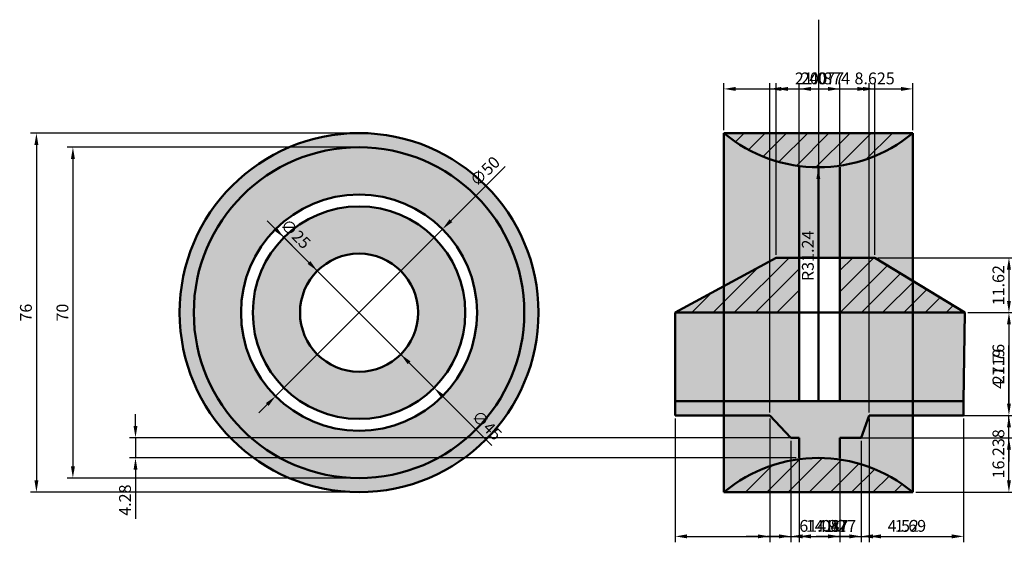
# Model space of a CAD drawing. Units: millimetres. Extents: x 1248 to 2192, y 1962 to 2325.
# Tile 1 of 4: x 1249 to 1457, y 1962 to 2073. Entities that reach past the tile are written whole.
import ezdxf

# ---------------------------------------------------------------- set-up
doc = ezdxf.new("R2010")
doc.units = ezdxf.units.MM
for name, color, linetype, lineweight in [('M-DIMS', 2, 'Continuous', 25), ('M-HATC', 8, 'Continuous', 18), ('M-OUTL', 7, 'Continuous', 50)]:
    doc.layers.add(name, color=color, linetype=linetype, lineweight=lineweight)
doc.styles.get("Standard").update_dxf_attribs({"font": 'arial.ttf'})
doc.dimstyles.new('ISO-25', dxfattribs={"dimtxt": 2.5, "dimasz": 2.5, "dimexe": 1.25, "dimexo": 0.625, "dimtad": 1, "dimtxsty": 'Standard', "dimcen": 2.5, "dimadec": 0, "dimazin": 0, "dimtfac": 1, "dimtmove": 0, "dimatfit": 3, "dimfxl": 1, "dimarcsym": 0})

# ---------------------------------------------------------------- blocks, each defined once
blk = doc.blocks.new('*D10')
at = {"layer": 'Defpoints', "color": 0, "transparency": 16777216}
for p in [(1320.58, 2048.72), (1252.24, 1972.72), (1320.58, 1972.72)]:
    blk.add_point(p, dxfattribs=at)
at = {"layer": 'M-DIMS', "color": 0, "lineweight": -2, "transparency": 16777216}
for p, q in [((1319.95, 2048.72), (1250.99, 2048.72)), ((1252.24, 2046.22), (1252.24, 1975.22)), ((1319.95, 1972.72), (1250.99, 1972.72))]:
    blk.add_line(p, q, dxfattribs=at)
at = {"layer": 'M-DIMS', "color": 0, "transparency": 16777216}
for points in [[(1251.82, 2046.22), (1252.66, 2046.22), (1252.24, 2048.72)], [(1251.82, 1975.22), (1252.66, 1975.22), (1252.24, 1972.72)]]:
    blk.add_solid(points, dxfattribs=at)
at = {"layer": 'M-DIMS', "color": 0, "transparency": 16777216, "insert": (1250.34, 2010.72), "char_height": 2.5, "attachment_point": 5, "rotation": 90}
blk.add_mtext('76', dxfattribs=at)
blk = doc.blocks.new('*D11')
at = {"layer": 'Defpoints', "color": 0, "transparency": 16777216}
for p in [(1320.58, 2045.72), (1259.97, 1975.72), (1320.58, 1975.72)]:
    blk.add_point(p, dxfattribs=at)
at = {"layer": 'M-DIMS', "color": 0, "lineweight": -2, "transparency": 16777216}
for p, q in [((1319.95, 2045.72), (1258.72, 2045.72)), ((1259.97, 2043.22), (1259.97, 1978.22)), ((1319.95, 1975.72), (1258.72, 1975.72))]:
    blk.add_line(p, q, dxfattribs=at)
at = {"layer": 'M-DIMS', "color": 0, "transparency": 16777216}
for points in [[(1259.55, 2043.22), (1260.39, 2043.22), (1259.97, 2045.72)], [(1259.55, 1978.22), (1260.39, 1978.22), (1259.97, 1975.72)]]:
    blk.add_solid(points, dxfattribs=at)
at = {"layer": 'M-DIMS', "color": 0, "transparency": 16777216, "insert": (1258.07, 2010.72), "char_height": 2.5, "attachment_point": 5, "rotation": 90}
blk.add_mtext('70', dxfattribs=at)
blk = doc.blocks.new('*D41')
at = {"layer": 'Defpoints', "color": 0, "transparency": 16777216}
for p in [(1437.87, 2058.07), (1397.87, 2048.72), (1437.87, 2048.72)]:
    blk.add_point(p, dxfattribs=at)
at = {"layer": 'M-DIMS', "color": 0, "lineweight": -2, "transparency": 16777216}
for p, q in [((1397.87, 2049.34), (1397.87, 2059.32)), ((1437.87, 2049.34), (1437.87, 2059.32)), ((1400.37, 2058.07), (1435.37, 2058.07))]:
    blk.add_line(p, q, dxfattribs=at)
at = {"layer": 'M-DIMS', "color": 0, "transparency": 16777216}
for points in [[(1400.37, 2058.49), (1400.37, 2057.65), (1397.87, 2058.07)], [(1435.37, 2058.49), (1435.37, 2057.65), (1437.87, 2058.07)]]:
    blk.add_solid(points, dxfattribs=at)
at = {"layer": 'M-DIMS', "color": 0, "transparency": 16777216, "insert": (1417.87, 2059.97), "char_height": 2.5, "attachment_point": 5}
blk.add_mtext('40', dxfattribs=at)
blk = doc.blocks.new('*D42')
at = {"layer": 'Defpoints', "color": 0, "transparency": 16777216}
for p in [(1387.56, 1988.96), (1448.64, 1988.96), (1448.64, 1963.37)]:
    blk.add_point(p, dxfattribs=at)
at = {"layer": 'M-DIMS', "color": 0, "lineweight": -2, "transparency": 16777216}
for p, q in [((1387.56, 1988.33), (1387.56, 1962.12)), ((1448.64, 1988.33), (1448.64, 1962.12)), ((1390.06, 1963.37), (1446.14, 1963.37))]:
    blk.add_line(p, q, dxfattribs=at)
at = {"layer": 'M-DIMS', "color": 0, "transparency": 16777216}
for points in [[(1390.06, 1963.79), (1390.06, 1962.95), (1387.56, 1963.37)], [(1446.14, 1963.79), (1446.14, 1962.95), (1448.64, 1963.37)]]:
    blk.add_solid(points, dxfattribs=at)
at = {"layer": 'M-DIMS', "color": 0, "transparency": 16777216, "insert": (1418.1, 1965.27), "char_height": 2.5, "attachment_point": 5}
blk.add_mtext('61.08', dxfattribs=at)
blk = doc.blocks.new('*D43')
at = {"layer": 'Defpoints', "color": 0, "transparency": 16777216}
for p in [(1448.89, 2010.72), (1448.64, 1988.96), (1458.24, 1988.96)]:
    blk.add_point(p, dxfattribs=at)
at = {"layer": 'M-DIMS', "color": 0, "lineweight": -2, "transparency": 16777216}
for p, q in [((1449.52, 2010.72), (1459.49, 2010.72)), ((1458.24, 2008.22), (1458.24, 1991.46)), ((1449.26, 1988.96), (1459.49, 1988.96))]:
    blk.add_line(p, q, dxfattribs=at)
at = {"layer": 'M-DIMS', "color": 0, "transparency": 16777216}
for points in [[(1457.83, 2008.22), (1458.66, 2008.22), (1458.24, 2010.72)], [(1457.83, 1991.46), (1458.66, 1991.46), (1458.24, 1988.96)]]:
    blk.add_solid(points, dxfattribs=at)
at = {"layer": 'M-DIMS', "color": 0, "transparency": 16777216, "insert": (1456.34, 1999.84), "char_height": 2.5, "attachment_point": 5, "rotation": 90}
blk.add_mtext('21.76', dxfattribs=at)
blk = doc.blocks.new('*D44')
at = {"layer": 'Defpoints', "color": 0, "transparency": 16777216}
for p in [(1429.82, 2022.34), (1448.89, 2010.72), (1458.24, 2010.72)]:
    blk.add_point(p, dxfattribs=at)
at = {"layer": 'M-DIMS', "color": 0, "lineweight": -2, "transparency": 16777216}
for p, q in [((1430.45, 2022.34), (1459.49, 2022.34)), ((1458.24, 2019.84), (1458.24, 2013.22)), ((1449.52, 2010.72), (1459.49, 2010.72))]:
    blk.add_line(p, q, dxfattribs=at)
at = {"layer": 'M-DIMS', "color": 0, "transparency": 16777216}
for points in [[(1457.83, 2019.84), (1458.66, 2019.84), (1458.24, 2022.34)], [(1457.83, 2013.22), (1458.66, 2013.22), (1458.24, 2010.72)]]:
    blk.add_solid(points, dxfattribs=at)
at = {"layer": 'M-DIMS', "color": 0, "transparency": 16777216, "insert": (1456.34, 2016.53), "char_height": 2.5, "attachment_point": 5, "rotation": 90}
blk.add_mtext('11.62', dxfattribs=at)
blk = doc.blocks.new('*D45')
at = {"layer": 'Defpoints', "color": 0, "transparency": 16777216}
for p in [(1448.64, 1988.96), (1458.24, 1988.96), (1437.87, 1972.72)]:
    blk.add_point(p, dxfattribs=at)
at = {"layer": 'M-DIMS', "color": 0, "lineweight": -2, "transparency": 16777216}
for p, q in [((1449.26, 1988.96), (1459.49, 1988.96)), ((1458.24, 1975.22), (1458.24, 1986.46)), ((1438.49, 1972.72), (1459.49, 1972.72))]:
    blk.add_line(p, q, dxfattribs=at)
at = {"layer": 'M-DIMS', "color": 0, "transparency": 16777216}
for points in [[(1457.83, 1986.46), (1458.66, 1986.46), (1458.24, 1988.96)], [(1457.83, 1975.22), (1458.66, 1975.22), (1458.24, 1972.72)]]:
    blk.add_solid(points, dxfattribs=at)
at = {"layer": 'M-DIMS', "color": 0, "transparency": 16777216, "insert": (1456.34, 1980.84), "char_height": 2.5, "attachment_point": 5, "rotation": 90}
blk.add_mtext('16.238', dxfattribs=at)
blk = doc.blocks.new('*D46')
at = {"layer": 'Defpoints', "color": 0, "transparency": 16777216}
for p in [(1429.82, 2058.07), (1408.95, 2022.34), (1429.82, 2022.34)]:
    blk.add_point(p, dxfattribs=at)
at = {"layer": 'M-DIMS', "color": 0, "lineweight": -2, "transparency": 16777216}
for p, q in [((1408.95, 2022.97), (1408.95, 2059.32)), ((1429.82, 2022.97), (1429.82, 2059.32)), ((1411.45, 2058.07), (1427.32, 2058.07))]:
    blk.add_line(p, q, dxfattribs=at)
at = {"layer": 'M-DIMS', "color": 0, "transparency": 16777216}
for points in [[(1411.45, 2058.49), (1411.45, 2057.65), (1408.95, 2058.07)], [(1427.32, 2058.49), (1427.32, 2057.65), (1429.82, 2058.07)]]:
    blk.add_solid(points, dxfattribs=at)
at = {"layer": 'M-DIMS', "color": 0, "transparency": 16777216, "insert": (1419.39, 2059.97), "char_height": 2.5, "attachment_point": 5}
blk.add_mtext('20.874', dxfattribs=at)
blk = doc.blocks.new('*D47')
at = {"layer": 'Defpoints', "color": 0, "transparency": 16777216}
for p in [(1422.43, 2058.07), (1413.81, 2041.48), (1422.43, 2041.48)]:
    blk.add_point(p, dxfattribs=at)
at = {"layer": 'M-DIMS', "color": 0, "lineweight": -2, "transparency": 16777216}
for p, q in [((1413.81, 2042.1), (1413.81, 2059.32)), ((1422.43, 2042.1), (1422.43, 2059.32)), ((1416.31, 2058.07), (1419.93, 2058.07)), ((1422.43, 2058.07), (1434.64, 2058.07))]:
    blk.add_line(p, q, dxfattribs=at)
at = {"layer": 'M-DIMS', "color": 0, "transparency": 16777216}
for points in [[(1416.31, 2058.49), (1416.31, 2057.65), (1413.81, 2058.07)], [(1419.93, 2058.49), (1419.93, 2057.65), (1422.43, 2058.07)]]:
    blk.add_solid(points, dxfattribs=at)
at = {"layer": 'M-DIMS', "color": 0, "transparency": 16777216, "insert": (1429.79, 2059.97), "char_height": 2.5, "attachment_point": 5}
blk.add_mtext('8.625', dxfattribs=at)
blk = doc.blocks.new('*D48')
at = {"layer": 'Defpoints', "color": 0, "transparency": 16777216}
for p in [(1412.03, 1984.24), (1426.95, 1984.24), (1426.95, 1963.37)]:
    blk.add_point(p, dxfattribs=at)
at = {"layer": 'M-DIMS', "color": 0, "lineweight": -2, "transparency": 16777216}
for p, q in [((1412.03, 1983.61), (1412.03, 1962.12)), ((1426.95, 1983.61), (1426.95, 1962.12)), ((1414.53, 1963.37), (1424.45, 1963.37))]:
    blk.add_line(p, q, dxfattribs=at)
at = {"layer": 'M-DIMS', "color": 0, "transparency": 16777216}
for points in [[(1414.53, 1963.79), (1414.53, 1962.95), (1412.03, 1963.37)], [(1424.45, 1963.79), (1424.45, 1962.95), (1426.95, 1963.37)]]:
    blk.add_solid(points, dxfattribs=at)
at = {"layer": 'M-DIMS', "color": 0, "transparency": 16777216, "insert": (1419.49, 1965.27), "char_height": 2.5, "attachment_point": 5}
blk.add_mtext('14.92', dxfattribs=at)
blk = doc.blocks.new('*D49')
at = {"layer": 'Defpoints', "color": 0, "transparency": 16777216}
for p in [(1428.64, 1988.96), (1458.24, 1988.96), (1422.43, 1984.24)]:
    blk.add_point(p, dxfattribs=at)
at = {"layer": 'M-DIMS', "color": 0, "lineweight": -2, "transparency": 16777216}
for p, q in [((1458.24, 1991.46), (1458.24, 2003.75)), ((1429.26, 1988.96), (1459.49, 1988.96)), ((1458.24, 1984.24), (1458.24, 1988.96)), ((1423.06, 1984.24), (1459.49, 1984.24)), ((1458.24, 1981.74), (1458.24, 1979.24))]:
    blk.add_line(p, q, dxfattribs=at)
at = {"layer": 'M-DIMS', "color": 0, "transparency": 16777216}
for points in [[(1457.83, 1991.46), (1458.66, 1991.46), (1458.24, 1988.96)], [(1457.83, 1981.74), (1458.66, 1981.74), (1458.24, 1984.24)]]:
    blk.add_solid(points, dxfattribs=at)
at = {"layer": 'M-DIMS', "color": 0, "transparency": 16777216, "insert": (1456.34, 1998.85), "char_height": 2.5, "attachment_point": 5, "rotation": 90}
blk.add_mtext('4.719', dxfattribs=at)
blk = doc.blocks.new('*D61')
at = {"layer": 'Defpoints', "color": 0, "transparency": 16777216}
for p in [(1338.26, 2028.4), (1302.9, 1993.04)]:
    blk.add_point(p, dxfattribs=at)
at = {"layer": 'M-DIMS', "color": 0, "lineweight": -2, "transparency": 16777216}
for p, q in [((1351.53, 2041.67), (1340.02, 2030.16)), ((1302.9, 1993.04), (1338.26, 2028.4)), ((1301.13, 1991.28), (1299.36, 1989.51))]:
    blk.add_line(p, q, dxfattribs=at)
at = {"layer": 'M-DIMS', "color": 0, "transparency": 16777216}
for points in [[(1339.73, 2030.46), (1340.32, 2029.87), (1338.26, 2028.4)], [(1300.83, 1991.57), (1301.42, 1990.98), (1302.9, 1993.04)]]:
    blk.add_solid(points, dxfattribs=at)
at = {"layer": 'M-DIMS', "color": 0, "transparency": 16777216, "insert": (1347.47, 2040.4), "char_height": 2.5, "attachment_point": 5, "rotation": 44.9946}
blk.add_mtext('∅50', dxfattribs=at)
blk = doc.blocks.new('*D62')
at = {"layer": 'Defpoints', "color": 0, "transparency": 16777216}
for p in [(1304.66, 2026.63), (1336.49, 1994.81)]:
    blk.add_point(p, dxfattribs=at)
at = {"layer": 'M-DIMS', "color": 0, "lineweight": -2, "transparency": 16777216}
for p, q in [((1302.9, 2028.4), (1301.13, 2030.16)), ((1304.66, 2026.63), (1336.49, 1994.81)), ((1348.71, 1982.59), (1338.26, 1993.04))]:
    blk.add_line(p, q, dxfattribs=at)
at = {"layer": 'M-DIMS', "color": 0, "transparency": 16777216}
for points in [[(1303.19, 2028.69), (1302.6, 2028.1), (1304.66, 2026.63)], [(1338.55, 1993.34), (1337.96, 1992.75), (1336.49, 1994.81)]]:
    blk.add_solid(points, dxfattribs=at)
at = {"layer": 'M-DIMS', "color": 0, "transparency": 16777216, "insert": (1347.43, 1986.66), "char_height": 2.5, "attachment_point": 5, "rotation": 315.0063}
blk.add_mtext('∅45', dxfattribs=at)
blk = doc.blocks.new('*D63')
at = {"layer": 'Defpoints', "color": 0, "transparency": 16777216}
for p in [(1311.74, 2019.56), (1329.41, 2001.88)]:
    blk.add_point(p, dxfattribs=at)
at = {"layer": 'M-DIMS', "color": 0, "lineweight": -2, "transparency": 16777216}
for p, q in [((1302.85, 2028.45), (1309.97, 2021.33)), ((1329.41, 2001.88), (1311.74, 2019.56)), ((1331.18, 2000.11), (1332.95, 1998.34))]:
    blk.add_line(p, q, dxfattribs=at)
at = {"layer": 'M-DIMS', "color": 0, "transparency": 16777216}
for points in [[(1310.27, 2021.62), (1309.68, 2021.03), (1311.74, 2019.56)], [(1331.48, 2000.41), (1330.89, 1999.82), (1329.41, 2001.88)]]:
    blk.add_solid(points, dxfattribs=at)
at = {"layer": 'M-DIMS', "color": 0, "transparency": 16777216, "insert": (1306.92, 2027.17), "char_height": 2.5, "attachment_point": 5, "rotation": 314.9886}
blk.add_mtext('∅25', dxfattribs=at)
blk = doc.blocks.new('*D64')
at = {"layer": 'Defpoints', "color": 0, "transparency": 16777216}
for p in [(1417.87, 2072.72), (1417.87, 2041.48)]:
    blk.add_point(p, dxfattribs=at)
at = {"layer": 'M-DIMS', "color": 0, "lineweight": -2, "transparency": 16777216}
for p, q in [((1417.87, 2072.72), (1417.87, 2041.48)), ((1417.87, 2016.7), (1417.87, 2038.98))]:
    blk.add_line(p, q, dxfattribs=at)
at = {"layer": 'M-DIMS', "color": 0, "transparency": 16777216}
blk.add_solid([(1417.45, 2038.98), (1418.28, 2038.98), (1417.87, 2041.48)], dxfattribs=at)
at = {"layer": 'M-DIMS', "color": 0, "transparency": 16777216, "insert": (1415.97, 2022.74), "char_height": 2.5, "attachment_point": 5, "rotation": 89.9997}
blk.add_mtext('R31.24', dxfattribs=at)
blk = doc.blocks.new('*D69')
at = {"layer": 'Defpoints', "color": 0, "transparency": 16777216}
for p in [(1428.64, 2058.07), (1407.56, 1988.96), (1428.64, 1988.96)]:
    blk.add_point(p, dxfattribs=at)
at = {"layer": 'M-DIMS', "color": 0, "lineweight": -2, "transparency": 16777216}
for p, q in [((1407.56, 1989.58), (1407.56, 2059.32)), ((1428.64, 1989.58), (1428.64, 2059.32)), ((1410.06, 2058.07), (1426.14, 2058.07))]:
    blk.add_line(p, q, dxfattribs=at)
at = {"layer": 'M-DIMS', "color": 0, "transparency": 16777216}
for points in [[(1410.06, 2058.49), (1410.06, 2057.65), (1407.56, 2058.07)], [(1426.14, 2058.49), (1426.14, 2057.65), (1428.64, 2058.07)]]:
    blk.add_solid(points, dxfattribs=at)
at = {"layer": 'M-DIMS', "color": 0, "transparency": 16777216, "insert": (1418.1, 2059.97), "char_height": 2.5, "attachment_point": 5}
blk.add_mtext('21.077', dxfattribs=at)
blk = doc.blocks.new('*D70')
at = {"layer": 'Defpoints', "color": 0, "transparency": 16777216}
for p in [(1407.56, 1988.96), (1412.03, 1984.24), (1412.03, 1963.37)]:
    blk.add_point(p, dxfattribs=at)
at = {"layer": 'M-DIMS', "color": 0, "lineweight": -2, "transparency": 16777216}
for p, q in [((1407.56, 1988.33), (1407.56, 1962.12)), ((1412.03, 1983.61), (1412.03, 1962.12)), ((1405.06, 1963.37), (1402.56, 1963.37)), ((1407.56, 1963.37), (1412.03, 1963.37)), ((1414.53, 1963.37), (1424.88, 1963.37))]:
    blk.add_line(p, q, dxfattribs=at)
at = {"layer": 'M-DIMS', "color": 0, "transparency": 16777216}
for points in [[(1405.06, 1963.79), (1405.06, 1962.95), (1407.56, 1963.37)], [(1414.53, 1963.79), (1414.53, 1962.95), (1412.03, 1963.37)]]:
    blk.add_solid(points, dxfattribs=at)
at = {"layer": 'M-DIMS', "color": 0, "transparency": 16777216, "insert": (1420.95, 1965.24), "char_height": 2.5, "attachment_point": 5}
blk.add_mtext('4.47', dxfattribs=at)
blk = doc.blocks.new('*D71')
at = {"layer": 'Defpoints', "color": 0, "transparency": 16777216}
for p in [(1412.03, 1984.24), (1413.81, 1984.24), (1413.81, 1963.37)]:
    blk.add_point(p, dxfattribs=at)
at = {"layer": 'M-DIMS', "color": 0, "lineweight": -2, "transparency": 16777216}
for p, q in [((1412.03, 1983.61), (1412.03, 1962.12)), ((1413.81, 1983.61), (1413.81, 1962.12)), ((1409.53, 1963.37), (1407.03, 1963.37)), ((1412.03, 1963.37), (1413.81, 1963.37)), ((1416.31, 1963.37), (1426.31, 1963.37))]:
    blk.add_line(p, q, dxfattribs=at)
at = {"layer": 'M-DIMS', "color": 0, "transparency": 16777216}
for points in [[(1409.53, 1963.79), (1409.53, 1962.95), (1412.03, 1963.37)], [(1416.31, 1963.79), (1416.31, 1962.95), (1413.81, 1963.37)]]:
    blk.add_solid(points, dxfattribs=at)
at = {"layer": 'M-DIMS', "color": 0, "transparency": 16777216, "insert": (1422.56, 1965.25), "char_height": 2.5, "attachment_point": 5}
blk.add_mtext('1.77', dxfattribs=at)
blk = doc.blocks.new('*D72')
at = {"layer": 'Defpoints', "color": 0, "transparency": 16777216}
for p in [(1422.43, 1984.24), (1426.95, 1984.24), (1426.95, 1963.37)]:
    blk.add_point(p, dxfattribs=at)
at = {"layer": 'M-DIMS', "color": 0, "lineweight": -2, "transparency": 16777216}
for p, q in [((1422.43, 1983.61), (1422.43, 1962.12)), ((1426.95, 1983.61), (1426.95, 1962.12)), ((1419.93, 1963.37), (1417.43, 1963.37)), ((1422.43, 1963.37), (1426.95, 1963.37)), ((1429.45, 1963.37), (1439.77, 1963.37))]:
    blk.add_line(p, q, dxfattribs=at)
at = {"layer": 'M-DIMS', "color": 0, "transparency": 16777216}
for points in [[(1419.93, 1963.79), (1419.93, 1962.95), (1422.43, 1963.37)], [(1429.45, 1963.79), (1429.45, 1962.95), (1426.95, 1963.37)]]:
    blk.add_solid(points, dxfattribs=at)
at = {"layer": 'M-DIMS', "color": 0, "transparency": 16777216, "insert": (1435.86, 1965.27), "char_height": 2.5, "attachment_point": 5}
blk.add_mtext('4.52', dxfattribs=at)
blk = doc.blocks.new('*D73')
at = {"layer": 'Defpoints', "color": 0, "transparency": 16777216}
for p in [(1428.64, 1988.96), (1426.95, 1984.24), (1428.64, 1963.37)]:
    blk.add_point(p, dxfattribs=at)
at = {"layer": 'M-DIMS', "color": 0, "lineweight": -2, "transparency": 16777216}
for p, q in [((1428.64, 1988.33), (1428.64, 1962.12)), ((1426.95, 1983.61), (1426.95, 1962.12)), ((1424.45, 1963.37), (1421.95, 1963.37)), ((1426.95, 1963.37), (1428.64, 1963.37)), ((1431.14, 1963.37), (1441.15, 1963.37))]:
    blk.add_line(p, q, dxfattribs=at)
at = {"layer": 'M-DIMS', "color": 0, "transparency": 16777216}
for points in [[(1424.45, 1963.79), (1424.45, 1962.95), (1426.95, 1963.37)], [(1431.14, 1963.79), (1431.14, 1962.95), (1428.64, 1963.37)]]:
    blk.add_solid(points, dxfattribs=at)
at = {"layer": 'M-DIMS', "color": 0, "transparency": 16777216, "insert": (1437.39, 1965.27), "char_height": 2.5, "attachment_point": 5}
blk.add_mtext('1.69', dxfattribs=at)
blk = doc.blocks.new('*D74')
at = {"layer": 'Defpoints', "color": 0, "transparency": 16777216}
for p in [(1413.81, 1984.24), (1273.23, 1979.96), (1413.81, 1979.96)]:
    blk.add_point(p, dxfattribs=at)
at = {"layer": 'M-DIMS', "color": 0, "lineweight": -2, "transparency": 16777216}
for p, q in [((1273.23, 1986.74), (1273.23, 1989.24)), ((1413.18, 1984.24), (1271.98, 1984.24)), ((1273.23, 1984.24), (1273.23, 1979.96)), ((1413.18, 1979.96), (1271.98, 1979.96)), ((1273.23, 1977.46), (1273.23, 1967.11))]:
    blk.add_line(p, q, dxfattribs=at)
at = {"layer": 'M-DIMS', "color": 0, "transparency": 16777216}
for points in [[(1272.81, 1986.74), (1273.64, 1986.74), (1273.23, 1984.24)], [(1272.81, 1977.46), (1273.64, 1977.46), (1273.23, 1979.96)]]:
    blk.add_solid(points, dxfattribs=at)
at = {"layer": 'M-DIMS', "color": 0, "transparency": 16777216, "insert": (1271.33, 1971.04), "char_height": 2.5, "attachment_point": 5, "rotation": 90}
blk.add_mtext('4.28', dxfattribs=at)

msp = doc.modelspace()

# ---------------------------------------------------------------- hatches: boundary and pattern name
at = {"layer": 'M-HATC'}
h = msp.add_hatch(color=256, dxfattribs=at)
h.set_gradient(color1=(255, 0, 0), color2=(255, 0, 0))
h.paths.add_polyline_path([(1285.5766, 2010.7199, 1), (1355.5766, 2010.7199, 1)], flags=0)
h.paths.add_polyline_path([(1345.5766, 2010.7199, -1), (1295.5766, 2010.7199, -1)], flags=0)
h.paths.add_polyline_path([(1343.0766, 2010.7199, -1), (1298.0766, 2010.7199, -1)], flags=0)
h.paths.add_polyline_path([(1333.0766, 2010.7199, -1), (1308.0766, 2010.7199, -1)], flags=0)
h.paths.add_polyline_path([(1282.5766, 2010.7199, 1), (1358.5766, 2010.7199, 1)])
h.paths.add_polyline_path([(1355.5766, 2010.7199, -1), (1285.5766, 2010.7199, -1)], flags=16)
h = msp.add_hatch(dxfattribs=at)
h.set_pattern_fill('ANSI31', color=256)
h.paths.add_polyline_path([(1437.8682, 2048.7199), (1397.8682, 2048.7199, 0.36209663)])
h.paths.add_polyline_path([(1397.8682, 1972.7199), (1437.8682, 1972.7199, 0.362065)])
h.paths.add_polyline_path([(1413.8061, 2022.341), (1408.9497, 2022.341), (1397.8682, 2016.3204), (1397.8682, 2010.7199), (1413.8061, 2010.7199)])
h.paths.add_polyline_path([(1437.8682, 2017.4391), (1429.824, 2022.341), (1422.4308, 2022.341), (1422.4308, 2010.7199), (1437.8682, 2010.7199)])
h.paths.add_polyline_path([(1437.8682, 2017.4391), (1437.8682, 2010.7199), (1448.8945, 2010.7199)])
h.paths.add_polyline_path([(1397.8682, 2016.3204), (1387.5598, 2010.7199), (1397.8682, 2010.7199)])
h = msp.add_hatch(color=256, dxfattribs=at)
h.set_gradient(color1=(255, 0, 0), color2=(255, 0, 0))
h.paths.add_polyline_path([(1437.8682, 2048.7199), (1397.8682, 2048.7199, 0.36209663)])
h.paths.add_polyline_path([(1397.8682, 1972.7199), (1437.8682, 1972.7199, 0.362065)], flags=17)
h.paths.add_polyline_path([(1437.8682, 2048.7199, -0.17547366), (1417.8682, 2041.478), (1417.8682, 2022.341), (1429.824, 2022.341), (1437.8682, 2017.4391)])
h.paths.add_polyline_path([(1417.8682, 2041.478, -0.17547366), (1397.8682, 2048.7199), (1397.8682, 2016.3204), (1408.9497, 2022.341), (1417.8682, 2022.341)])
h.paths.add_polyline_path([(1413.8061, 2010.7199), (1397.8682, 2010.7199), (1397.8682, 1991.958), (1413.8061, 1991.958)])
h.paths.add_polyline_path([(1437.8682, 2010.7199), (1422.4308, 2010.7199), (1422.4308, 1991.958), (1437.8682, 1991.958)])
h.paths.add_polyline_path([(1437.8682, 2017.4391), (1429.824, 2022.341), (1422.4308, 2022.341), (1422.4308, 2010.7199), (1437.8682, 2010.7199)])
h.paths.add_polyline_path([(1413.8061, 2022.341), (1408.9497, 2022.341), (1397.8682, 2016.3204), (1397.8682, 2010.7199), (1413.8061, 2010.7199)])
h.paths.add_polyline_path([(1397.8682, 2016.3204), (1387.5598, 2010.7199), (1397.8682, 2010.7199)])
h.paths.add_polyline_path([(1437.8682, 2017.4391), (1437.8682, 2010.7199), (1448.8945, 2010.7199)])
h.paths.add_polyline_path([(1437.8682, 1991.958), (1422.4308, 1991.958), (1397.8682, 1991.958), (1397.8682, 1972.7199, -0.362065), (1437.8682, 1972.7199)])
h.paths.add_polyline_path([(1397.8682, 1991.958), (1387.5598, 1991.958), (1387.5598, 1988.958), (1397.8682, 1988.958)])
h.paths.add_polyline_path([(1448.6368, 1991.958), (1437.8682, 1991.958), (1437.8682, 1988.958), (1448.6368, 1988.958)])
h.paths.add_polyline_path([(1397.8682, 2010.7199), (1387.5598, 2010.7199), (1387.5598, 1991.958), (1397.8682, 1991.958)])
h = msp.add_hatch(color=256, dxfattribs=at)
h.set_gradient(color1=(255, 0, 0), color2=(255, 0, 0))
h.paths.add_polyline_path([(1437.8682, 1991.958), (1448.6368, 1991.958), (1448.8945, 2010.7199), (1437.8682, 2010.7199)])

# ---------------------------------------------------------------- linework, layer by layer
at = {"layer": 'M-OUTL'}
for p, q in [((1397.8682, 2048.7199), (1397.8682, 1972.7199)), ((1437.8682, 2048.7199), (1397.8682, 2048.7199)), ((1437.8682, 1972.7199), (1437.8682, 2048.7199)), ((1413.8061, 2041.478), (1413.8061, 1991.958)), ((1417.8682, 2041.478), (1417.8682, 1991.958)), ((1422.4308, 2041.478), (1422.4308, 1991.958)), ((1408.9497, 2022.341), (1387.5598, 2010.7199)), ((1408.9497, 2022.341), (1429.824, 2022.341)), ((1429.824, 2022.341), (1448.8945, 2010.7199)), ((1397.8682, 2010.7199), (1387.5598, 2010.7199)), ((1387.5598, 2010.7199), (1448.8945, 2010.7199)), ((1387.5598, 2010.7199), (1387.5598, 1991.958)), ((1448.8945, 2010.7199), (1448.6368, 1991.958)), ((1387.5598, 1991.958), (1448.6368, 1991.958)), ((1387.5598, 1991.958), (1387.5598, 1988.958)), ((1448.6368, 1991.958), (1448.6368, 1988.958)), ((1387.5598, 1988.958), (1407.5598, 1988.958)), ((1407.5598, 1988.958), (1412.0314, 1984.2387)), ((1426.9503, 1984.2387), (1428.6368, 1988.958)), ((1448.6368, 1988.958), (1428.6368, 1988.958)), ((1412.0314, 1984.2387), (1413.8061, 1984.2387)), ((1413.8061, 1984.2387), (1413.8061, 1979.9612)), ((1422.4308, 1984.2387), (1426.9503, 1984.2387)), ((1422.4308, 1984.2387), (1422.4308, 1979.9612)), ((1397.8682, 1972.7199), (1437.8682, 1972.7199))]:
    msp.add_line(p, q, dxfattribs=at)
for radius in [38, 35, 25, 22.5, 12.5]:
    msp.add_circle((1320.5766, 2010.7199), radius, dxfattribs=at)
for centre, radius, start, end in [((1417.8682, 2072.7159), 31.2379, 230.189698, 309.810302), ((1417.8682, 1948.7212), 31.24, 50.192902, 129.807098)]:
    msp.add_arc(centre, radius, start, end, dxfattribs=at)

# ---------------------------------------------------------------- dimensions: what is measured, and where the dimension line sits
at = {"layer": 'M-DIMS'}
dim = msp.add_radius_dim(center=(1417.8682, 2072.7159), mpoint=(1417.868, 2041.478), dimstyle='ISO-25', override={"dimdec": 2, "dimlfac": 1, "dimrnd": 0, "dimzin": 0, "dimdsep": 46, "dimlunit": 2}, dxfattribs=at)
dim.commit()
dim.dimension.update_dxf_attribs({"geometry": '*D64', "text_midpoint": (1417.8679, 2022.7352), "dimtype": 164})
for base, p1, p2, override, picture, middle in [((1437.8682, 2058.0699), (1397.8682, 2048.7199), (1437.8682, 2048.7199), {"dimdec": 0, "dimlfac": 1, "dimrnd": 0, "dimzin": 0, "dimdsep": 46, "dimlunit": 2}, '*D41', (1417.8682, 2059.9713)), ((1428.6368, 2058.0699), (1407.5598, 1988.958), (1428.6368, 1988.958), {"dimdec": 3, "dimlfac": 1, "dimrnd": 0, "dimzin": 0, "dimdsep": 46, "dimlunit": 2}, '*D69', (1418.0983, 2059.9713)), ((1429.824, 2058.0699), (1408.9497, 2022.341), (1429.824, 2022.341), {"dimdec": 3, "dimlfac": 1, "dimrnd": 0, "dimzin": 0, "dimdsep": 46, "dimlunit": 2}, '*D46', (1419.3868, 2059.9713)), ((1422.4308, 2058.0699), (1413.8061, 2041.478), (1422.4308, 2041.478), {"dimdec": 3, "dimlfac": 1, "dimrnd": 0, "dimzin": 0, "dimdsep": 46, "dimlunit": 2}, '*D47', (1429.785, 2059.9713)), ((1448.6368, 1963.3699), (1387.5598, 1988.958), (1448.6368, 1988.958), {"dimdec": 2, "dimlfac": 1, "dimrnd": 0, "dimzin": 0, "dimdsep": 46, "dimlunit": 2}, '*D42', (1418.0983, 1965.2713)), ((1412.0314, 1963.3699), (1407.5598, 1988.958), (1412.0314, 1984.2387), {"dimdec": 2, "dimlfac": 1, "dimrnd": 0, "dimzin": 0, "dimdsep": 46, "dimlunit": 2}, '*D70', (1420.9536, 1965.2449)), ((1428.6368, 1963.3699), (1426.9503, 1984.2387), (1428.6368, 1988.958), {"dimdec": 2, "dimlfac": 1, "dimrnd": 0, "dimzin": 0, "dimdsep": 46, "dimlunit": 2}, '*D73', (1437.3936, 1965.2713)), ((1413.8061, 1963.3699), (1412.0314, 1984.2387), (1413.8061, 1984.2387), {"dimdec": 2, "dimlfac": 1, "dimrnd": 0, "dimzin": 0, "dimdsep": 46, "dimlunit": 2}, '*D71', (1422.5603, 1965.25)), ((1426.9503, 1963.3699), (1412.0314, 1984.2387), (1426.9503, 1984.2387), {"dimdec": 2, "dimlfac": 1, "dimrnd": 0, "dimzin": 0, "dimdsep": 46, "dimlunit": 2}, '*D48', (1419.4908, 1965.2713)), ((1426.9503, 1963.3699), (1422.4308, 1984.2387), (1426.9503, 1984.2387), {"dimdec": 2, "dimlfac": 1, "dimrnd": 0, "dimzin": 0, "dimdsep": 46, "dimlunit": 2}, '*D72', (1435.8597, 1965.2713))]:
    dim = msp.add_linear_dim(base=base, p1=p1, p2=p2, dimstyle='ISO-25', override=override, dxfattribs=at)
    dim.commit()
    dim.dimension.update_dxf_attribs({"geometry": picture, "text_midpoint": middle})
for base, p1, p2, override, picture, middle in [((1252.2403, 1972.7199), (1320.5766, 2048.7199), (1320.5766, 1972.7199), {"dimclrd": 0, "dimclre": 0, "dimclrt": 0}, '*D10', (1250.3388, 2010.7199)), ((1259.9715, 1975.7199), (1320.5766, 2045.7199), (1320.5766, 1975.7199), {"dimclrd": 0, "dimclre": 0, "dimclrt": 0}, '*D11', (1258.0701, 2010.7199)), ((1458.2445, 2010.7199), (1429.824, 2022.341), (1448.8945, 2010.7199), {"dimdec": 2, "dimlfac": 1, "dimrnd": 0, "dimzin": 0, "dimdsep": 46, "dimlunit": 2}, '*D44', (1456.3431, 2016.5305)), ((1458.2445, 1988.958), (1448.8945, 2010.7199), (1448.6368, 1988.958), {"dimdec": 2, "dimlfac": 1, "dimrnd": 0, "dimzin": 0, "dimdsep": 46, "dimlunit": 2}, '*D43', (1456.3431, 1999.8389)), ((1458.2445, 1988.958), (1422.4308, 1984.2387), (1428.6368, 1988.958), {"dimdec": 3, "dimlfac": 1, "dimrnd": 0, "dimzin": 0, "dimdsep": 46, "dimlunit": 2}, '*D49', (1456.3431, 1998.854)), ((1273.2266, 1979.9612), (1413.8061, 1984.2387), (1413.8061, 1979.9612), {"dimdec": 2, "dimlfac": 1, "dimrnd": 0, "dimzin": 0, "dimdsep": 46, "dimlunit": 2}, '*D74', (1271.3252, 1971.0364)), ((1458.2445, 1988.958), (1437.8682, 1972.7199), (1448.6368, 1988.958), {"dimdec": 3, "dimlfac": 1, "dimrnd": 0, "dimzin": 0, "dimdsep": 46, "dimlunit": 2}, '*D45', (1456.3422, 1980.8389))]:
    dim = msp.add_linear_dim(base=base, p1=p1, p2=p2, angle=90, dimstyle='ISO-25', override=override, dxfattribs=at)
    dim.commit()
    dim.dimension.update_dxf_attribs({"geometry": picture, "text_midpoint": middle})
for p1, p2, picture, middle in [((1302.8973, 1993.0439), (1338.2559, 2028.3959), '*D61', (1348.8635, 2039.0015)), ((1304.6649, 2026.6281), (1336.4882, 1994.8118), '*D62', (1346.0352, 1985.2669))]:
    dim = msp.add_diameter_dim_2p(p1=p1, p2=p2, dimstyle='ISO-25', override={"dimdec": 0, "dimlfac": 1, "dimrnd": 0, "dimzin": 0, "dimdsep": 46, "dimlunit": 2}, dxfattribs=at)
    dim.commit()
    dim.dimension.update_dxf_attribs({"geometry": picture, "text_midpoint": middle, "dimtype": 163})
dim = msp.add_diameter_dim_2p(p1=(1329.4137, 2001.8793), p2=(1311.7395, 2019.5605), dimstyle='ISO-25', override={"dimdec": 0, "dimlfac": 1, "dimrnd": 0, "dimzin": 0, "dimdsep": 46, "dimlunit": 2}, dxfattribs=at)
dim.commit()
dim.dimension.update_dxf_attribs({"geometry": '*D63', "text_midpoint": (1305.5288, 2025.7736)})

doc.saveas('drawing.dxf')
